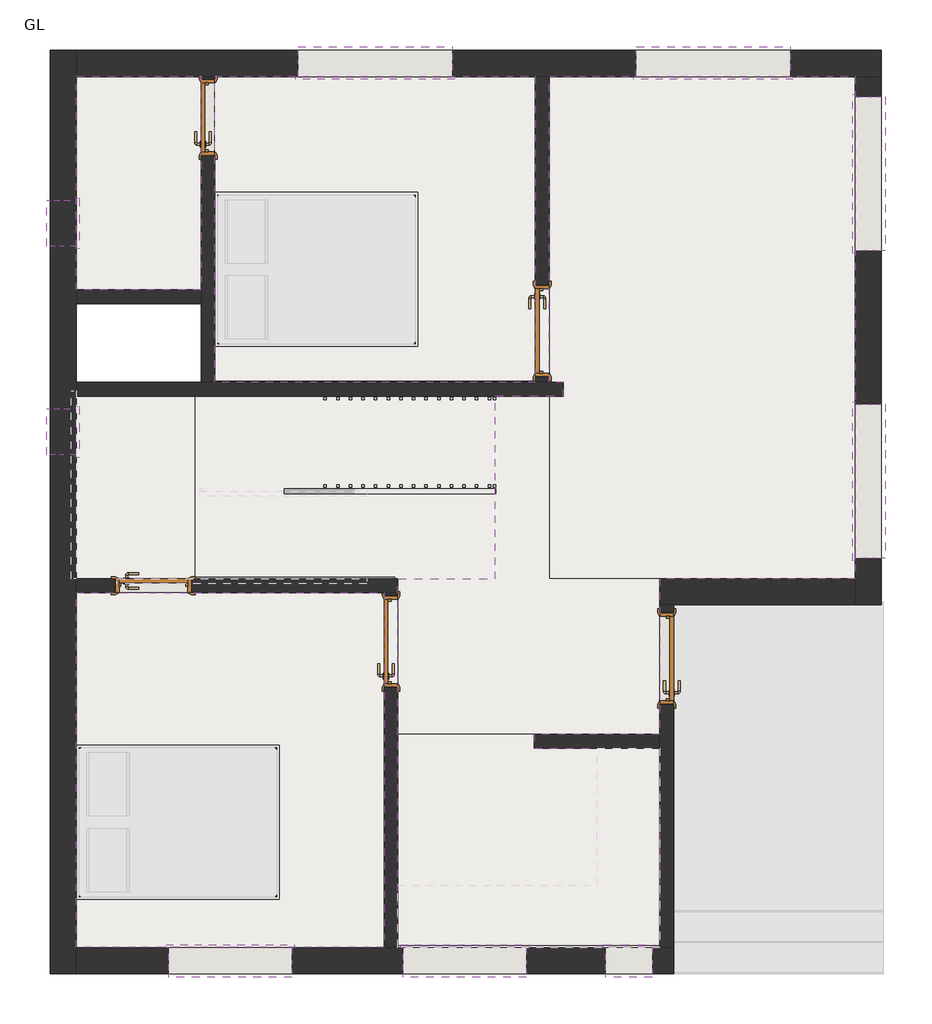
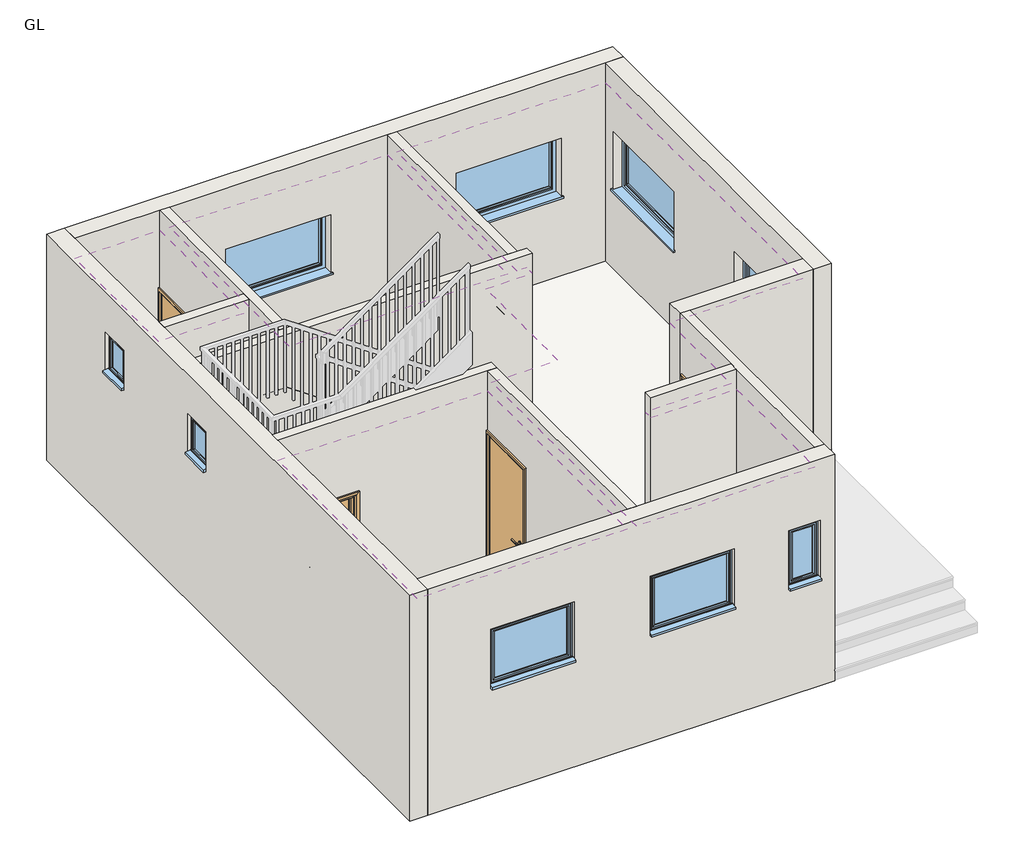
# One storey, part 1 of 2: 13 walls, 9 windows, 5 doors, 5 slabs, 4 coverings.
"""IFC4 building model written with IfcOpenShell, lengths in millimetres."""

from ifc_helpers import new_model, si_unit, frame, origin, origin_with_axes, place, context, project, spatial, polyline, outline, extrude, faceted_brep, transform, mapped, element, save
from components import doors_intsgl_d1_00c56c0f, doors_intsgl_d1_0ae72840, doors_intsgl_d2_4a296642, windows_sgl_plain_1219x910mm_2_5c67ae2b, windows_sgl_plain_w1_a675e60d, windows_sgl_plain_w3_7aa8ff83, windows_sgl_plain_w4_7e877f05

model = new_model("IFC4")

# Units and contexts
model_context = context("Model", 3, world=origin())
ifc_project = project(units=[si_unit("LENGTHUNIT", "METRE", prefix="MILLI")], contexts=[model_context])

# Site, building, storey
site = spatial("IfcSite", under=ifc_project)
building = spatial("IfcBuilding", under=site)
storey = spatial("IfcBuildingStorey", under=building, Name="GL", Elevation=0.0)

# Coverings
placement = place(None, origin())
element("IfcCovering", 1, ObjectType="Plain", at=placement, inside=storey, context=model_context, shape_type="SweptSolid", body=[
    extrude(outline(polyline([(-9804.9104231, 8478.0271174), (-11039.3504231, 8478.0271174), (-11039.3504231, 10590.7006314), (-9804.9104231, 10590.7006314), (-9804.9104231, 8478.0271174)])), frame((0.0, 0.0, 2743.2), z_axis=(0.0, 0.0, 1.0), x_axis=(1.0, 0.0, 0.0)), (0.0, 0.0, 1.0), 57.0),
])
element("IfcCovering", 2, ObjectType="Plain", at=placement, inside=storey, context=model_context, shape_type="SweptSolid", body=[
    extrude(outline(polyline([(-9667.7504231, 10590.7006314), (-6495.2904231, 10590.7006314), (-6495.2904231, 7563.6271174), (-9667.7504231, 7563.6271174), (-9667.7504231, 10590.7006314)])), frame((0.0, 0.0, 2743.2), z_axis=(0.0, 0.0, 1.0), x_axis=(1.0, 0.0, 0.0)), (0.0, 0.0, 1.0), 57.0),
])
element("IfcCovering", 3, ObjectType="Plain", at=placement, inside=storey, context=model_context, shape_type="SweptSolid", body=[
    extrude(outline(polyline([(-11039.3504231, 1964.8606314), (-11039.3504231, 5477.6191611), (-7992.723883, 5477.6191611), (-7992.723883, 1964.8606314), (-11039.3504231, 1964.8606314)])), frame((0.0, 0.0, 2743.2), z_axis=(0.0, 0.0, 1.0), x_axis=(1.0, 0.0, 0.0)), (0.0, 0.0, 1.0), 57.0),
])
element("IfcCovering", 4, ObjectType="Plain", at=placement, inside=storey, context=model_context, shape_type="SweptSolid", body=[
    extrude(outline(polyline([(-7855.563883, 1964.8606314), (-7855.563883, 5614.7791611), (-6892.1428068, 5614.7791611), (-6892.1428068, 7426.4671174), (-6216.8499038, 7426.4671174), (-6216.8499038, 7563.6271174), (-6358.1304231, 7563.6271174), (-6358.1304231, 10590.7006314), (-3327.9104231, 10590.7006314), (-3327.9104231, 5618.7656226), (-5262.223883, 5618.7656226), (-5262.223883, 4077.4180989), (-6506.823883, 4077.4180989), (-6506.823883, 3940.2580989), (-5262.223883, 3940.2580989), (-5262.223883, 1964.8606314), (-7855.563883, 1964.8606314)])), frame((0.0, 0.0, 2743.2), z_axis=(0.0, 0.0, 1.0), x_axis=(1.0, 0.0, 0.0)), (0.0, 0.0, 1.0), 57.0),
])

# Doors
doors_intsgl_d1_shape = doors_intsgl_d1_00c56c0f(model_context)
element("IfcDoor", 5, ObjectType="Doors_IntSgl : D1", at=placement, inside=storey, context=model_context, shape_type="MappedRepresentation", body=[
    mapped(doors_intsgl_d1_shape, transform((-6426.7104231, 8071.6271174, 0.0), x_axis=(0.0, -1.0, 0.0), y_axis=(1.0, 0.0, 0.0), z_axis=(0.0, 0.0, 1.0))),
])
element("IfcDoor", 6, ObjectType="Doors_IntSgl : D1", at=placement, inside=storey, context=model_context, shape_type="MappedRepresentation", body=[
    mapped(doors_intsgl_d1_shape, transform((-5193.643883, 4826.2856226, 0.0), x_axis=(0.0, 1.0, 0.0), y_axis=(-1.0, 0.0, 0.0), z_axis=(0.0, 0.0, 1.0))),
])
doors_intsgl_d1_2_shape = doors_intsgl_d1_0ae72840(model_context)
element("IfcDoor", 7, ObjectType="Doors_IntSgl : D1", at=placement, inside=storey, context=model_context, shape_type="MappedRepresentation", body=[
    mapped(doors_intsgl_d1_2_shape, transform((-7924.143883, 4995.0191611, 0.0), x_axis=(0.0, 1.0, 0.0), y_axis=(-1.0, 0.0, 0.0), z_axis=(0.0, 0.0, 1.0))),
])
doors_intsgl_d2_shape = doors_intsgl_d2_4a296642(model_context)
element("IfcDoor", 8, ObjectType="Doors_IntSgl : D2", at=placement, inside=storey, context=model_context, shape_type="MappedRepresentation", body=[
    mapped(doors_intsgl_d2_shape, transform((-10277.3504231, 5546.1991611, 0.0), x_axis=(1.0, 0.0, 0.0), y_axis=(0.0, 1.0, 0.0), z_axis=(0.0, 0.0, 1.0))),
])
element("IfcDoor", 9, ObjectType="Doors_IntSgl : D2", at=placement, inside=storey, context=model_context, shape_type="MappedRepresentation", body=[
    mapped(doors_intsgl_d2_shape, transform((-9736.3304231, 10185.6856226, 0.0), x_axis=(0.0, 1.0, 0.0), y_axis=(-1.0, 0.0, 0.0), z_axis=(0.0, 0.0, 1.0))),
])

# Slabs
element("IfcSlab", 10, ObjectType="BEDROOM FLOOR", at=placement, inside=storey, context=model_context, shape_type="SweptSolid", body=[
    extrude(outline(polyline([(-6358.1304231, 10590.7006314), (-6358.1304231, 7579.4271174), (-9667.7504231, 7579.4271174), (-9667.7504231, 10590.7006314), (-6358.1304231, 10590.7006314)])), origin_with_axes(), (0.0, 0.0, 1.0), 149.9616),
    extrude(outline(polyline([(-7855.563883, 5477.6191611), (-7855.563883, 1964.8606314), (-11039.3504231, 1964.8606314), (-11039.3504231, 5477.6191611), (-7855.563883, 5477.6191611)])), origin_with_axes(), (0.0, 0.0, 1.0), 149.9616),
])
element("IfcSlab", 11, ObjectType="FOYER", at=placement, inside=storey, context=model_context, shape_type="SweptSolid", body=[
    extrude(outline(polyline([(-5262.223883, 4077.4180989), (-7880.1504231, 4077.4180989), (-7880.1504231, 5634.7791611), (-9861.3504231, 5634.7791611), (-9861.3504231, 7426.4671174), (-6358.1304231, 7426.4671174), (-6358.1304231, 5618.7656226), (-5262.223883, 5618.7656226), (-5262.223883, 4077.4180989)])), frame((0.0, 0.0, -149.9616), z_axis=(0.0, 0.0, 1.0), x_axis=(1.0, 0.0, 0.0)), (0.0, 0.0, 1.0), 149.9616),
])
element("IfcSlab", 12, ObjectType="KITCHEN FLOOR", at=placement, inside=storey, context=model_context, shape_type="SweptSolid", body=[
    extrude(outline(polyline([(-7855.563883, 1989.8606314), (-7855.563883, 4077.4180989), (-5262.223883, 4077.4180989), (-5262.223883, 1989.8606314), (-7855.563883, 1989.8606314)])), frame((0.0, 0.0, -149.9616), z_axis=(0.0, 0.0, 1.0), x_axis=(1.0, 0.0, 0.0)), (0.0, 0.0, 1.0), 149.9616),
])
element("IfcSlab", 13, ObjectType="LIVING AND DINING AREA", at=placement, inside=storey, context=model_context, shape_type="SweptSolid", body=[
    extrude(outline(polyline([(-3327.9104231, 10590.7006314), (-3327.9104231, 5618.7656226), (-6358.1304231, 5618.7656226), (-6358.1304231, 10590.7006314), (-3327.9104231, 10590.7006314)])), frame((0.0, 0.0, -149.9616), z_axis=(0.0, 0.0, 1.0), x_axis=(1.0, 0.0, 0.0)), (0.0, 0.0, 1.0), 149.9616),
])
element("IfcSlab", 14, ObjectType="TOILET FLOOR", at=placement, inside=storey, context=model_context, shape_type="SweptSolid", body=[
    extrude(outline(polyline([(-9667.7504231, 10590.7006314), (-9667.7504231, 8478.0271174), (-11039.3504231, 8478.0271174), (-11039.3504231, 10590.7006314), (-9667.7504231, 10590.7006314)])), frame((0.0, 0.0, -149.9616), z_axis=(0.0, 0.0, 1.0), x_axis=(1.0, 0.0, 0.0)), (0.0, 0.0, 1.0), 149.9616),
    extrude(outline(polyline([(-9861.3504231, 7426.4671174), (-9861.3504231, 5477.6191611), (-11039.3504231, 5477.6191611), (-11039.3504231, 7426.4671174), (-9861.3504231, 7426.4671174)])), frame((0.0, 0.0, -149.9616), z_axis=(0.0, 0.0, 1.0), x_axis=(1.0, 0.0, 0.0)), (0.0, 0.0, 1.0), 149.9616),
])

# Walls
element("IfcWall", 15, ObjectType="EX WALL", at=placement, inside=storey, context=model_context, shape_type="Brep", body=[
    faceted_brep([(-11298.4304231, 10849.7806314, -426.72), (-11298.4304231, 1705.7806314, -426.72), (-11298.4304231, 1705.7806314, 3048.0), (-11298.4304231, 10849.7806314, 3048.0), (-11298.4304231, 6842.2671174, 2438.4), (-11298.4304231, 6842.2671174, 1828.8), (-11298.4304231, 7299.4671174, 1828.8), (-11298.4304231, 7299.4671174, 2438.4), (-11298.4304231, 8909.8271174, 2438.4), (-11298.4304231, 8909.8271174, 1828.8), (-11298.4304231, 9367.0271174, 1828.8), (-11298.4304231, 9367.0271174, 2438.4), (-11039.3504231, 10849.7806314, -426.72), (-11039.3504231, 10849.7806314, 3048.0), (-11039.3504231, 10590.7006314, 3048.0), (-11039.3504231, 8478.0271174, 3048.0), (-11039.3504231, 8340.8671174, 3048.0), (-11039.3504231, 7563.6271174, 3048.0), (-11039.3504231, 7426.4671174, 3048.0), (-11039.3504231, 5614.7791611, 3048.0), (-11039.3504231, 5477.6191611, 3048.0), (-11039.3504231, 1964.8606314, 3048.0), (-11039.3504231, 1705.7806314, 3048.0), (-11039.3504231, 1705.7806314, -426.72), (-11039.3504231, 1964.8606314, -426.72), (-11039.3504231, 5477.6191611, -426.72), (-11039.3504231, 5614.7791611, -426.72), (-11039.3504231, 7426.4671174, -426.72), (-11039.3504231, 7563.6271174, -426.72), (-11039.3504231, 8340.8671174, -426.72), (-11039.3504231, 8478.0271174, -426.72), (-11039.3504231, 10590.7006314, -426.72), (-11039.3504231, 6842.2671174, 2438.4), (-11039.3504231, 7299.4671174, 2438.4), (-11039.3504231, 7299.4671174, 1828.8), (-11039.3504231, 6842.2671174, 1828.8), (-11039.3504231, 8909.8271174, 2438.4), (-11039.3504231, 9367.0271174, 2438.4), (-11039.3504231, 9367.0271174, 1828.8), (-11039.3504231, 8909.8271174, 1828.8)], [[[0, 1, 2, 3], [4, 5, 6, 7], [8, 9, 10, 11]], [[12, 13, 14, 15, 16, 17, 18, 19, 20, 21, 22, 23, 24, 25, 26, 27, 28, 29, 30, 31], [32, 33, 34, 35], [36, 37, 38, 39]], [[1, 0, 12, 31, 30, 29, 28, 27, 26, 25, 24, 23]], [[3, 2, 22, 21, 20, 19, 18, 17, 16, 15, 14, 13]], [[2, 1, 23, 22]], [[0, 3, 13, 12]], [[5, 4, 32, 35]], [[6, 5, 35, 34]], [[7, 6, 34, 33]], [[4, 7, 33, 32]], [[9, 8, 36, 39]], [[10, 9, 39, 38]], [[11, 10, 38, 37]], [[8, 11, 37, 36]]]),
])
element("IfcWall", 16, ObjectType="EX WALL", at=placement, inside=storey, context=model_context, shape_type="Brep", body=[
    faceted_brep([(-5125.063883, 1964.8606314, -426.72), (-5262.223883, 1964.8606314, -426.72), (-7855.563883, 1964.8606314, -426.72), (-7992.723883, 1964.8606314, -426.72), (-11039.3504231, 1964.8606314, -426.72), (-11039.3504231, 1964.8606314, 3048.0), (-7992.723883, 1964.8606314, 3048.0), (-7855.563883, 1964.8606314, 3048.0), (-5262.223883, 1964.8606314, 3048.0), (-5125.063883, 1964.8606314, 3048.0), (-8906.4371531, 1964.8606314, 2110.0), (-10125.6371531, 1964.8606314, 2110.0), (-10125.6371531, 1964.8606314, 1200.0), (-8906.4371531, 1964.8606314, 1200.0), (-6585.563883, 1964.8606314, 2110.0), (-7804.763883, 1964.8606314, 2110.0), (-7804.763883, 1964.8606314, 1200.0), (-6585.563883, 1964.8606314, 1200.0), (-5338.423883, 1964.8606314, 2110.0), (-5795.623883, 1964.8606314, 2110.0), (-5795.623883, 1964.8606314, 1200.0), (-5338.423883, 1964.8606314, 1200.0), (-5125.063883, 1705.7806314, -426.72), (-5125.063883, 1705.7806314, 3048.0), (-11039.3504231, 1705.7806314, 3048.0), (-11039.3504231, 1705.7806314, -426.72), (-8906.4371531, 1705.7806314, 2110.0), (-8906.4371531, 1705.7806314, 1200.0), (-10125.6371531, 1705.7806314, 1200.0), (-10125.6371531, 1705.7806314, 2110.0), (-6585.563883, 1705.7806314, 2110.0), (-6585.563883, 1705.7806314, 1200.0), (-7804.763883, 1705.7806314, 1200.0), (-7804.763883, 1705.7806314, 2110.0), (-5338.423883, 1705.7806314, 2110.0), (-5338.423883, 1705.7806314, 1200.0), (-5795.623883, 1705.7806314, 1200.0), (-5795.623883, 1705.7806314, 2110.0)], [[[0, 1, 2, 3, 4, 5, 6, 7, 8, 9], [10, 11, 12, 13], [14, 15, 16, 17], [18, 19, 20, 21]], [[22, 23, 24, 25], [26, 27, 28, 29], [30, 31, 32, 33], [34, 35, 36, 37]], [[4, 3, 2, 1, 0, 22, 25]], [[9, 8, 7, 6, 5, 24, 23]], [[5, 4, 25, 24]], [[0, 9, 23, 22]], [[27, 26, 10, 13]], [[28, 27, 13, 12]], [[29, 28, 12, 11]], [[26, 29, 11, 10]], [[31, 30, 14, 17]], [[32, 31, 17, 16]], [[33, 32, 16, 15]], [[30, 33, 15, 14]], [[35, 34, 18, 21]], [[36, 35, 21, 20]], [[37, 36, 20, 19]], [[34, 37, 19, 18]]]),
])
element("IfcWall", 17, ObjectType="EX WALL", at=placement, inside=storey, context=model_context, shape_type="Brep", body=[
    faceted_brep([(-11039.3504231, 10590.7006314, -426.72), (-9804.9104231, 10590.7006314, -426.72), (-9667.7504231, 10590.7006314, -426.72), (-6495.2904231, 10590.7006314, -426.72), (-6358.1304231, 10590.7006314, -426.72), (-3327.9104231, 10590.7006314, -426.72), (-3068.8304231, 10590.7006314, -426.72), (-3068.8304231, 10590.7006314, 3048.0), (-3327.9104231, 10590.7006314, 3048.0), (-6358.1304231, 10590.7006314, 3048.0), (-6495.2904231, 10590.7006314, 3048.0), (-9667.7504231, 10590.7006314, 3048.0), (-9804.9104231, 10590.7006314, 3048.0), (-11039.3504231, 10590.7006314, 3048.0), (-8843.5204231, 10590.7006314, 2110.0), (-7319.5204231, 10590.7006314, 2110.0), (-7319.5204231, 10590.7006314, 1200.0), (-8843.5204231, 10590.7006314, 1200.0), (-5494.5304231, 10590.7006314, 2110.0), (-3970.5304231, 10590.7006314, 2110.0), (-3970.5304231, 10590.7006314, 1200.0), (-5494.5304231, 10590.7006314, 1200.0), (-11039.3504231, 10849.7806314, -426.72), (-11039.3504231, 10849.7806314, 3048.0), (-3068.8304231, 10849.7806314, 3048.0), (-3068.8304231, 10849.7806314, -426.72), (-8843.5204231, 10849.7806314, 2110.0), (-8843.5204231, 10849.7806314, 1200.0), (-7319.5204231, 10849.7806314, 1200.0), (-7319.5204231, 10849.7806314, 2110.0), (-5494.5304231, 10849.7806314, 2110.0), (-5494.5304231, 10849.7806314, 1200.0), (-3970.5304231, 10849.7806314, 1200.0), (-3970.5304231, 10849.7806314, 2110.0)], [[[0, 1, 2, 3, 4, 5, 6, 7, 8, 9, 10, 11, 12, 13], [14, 15, 16, 17], [18, 19, 20, 21]], [[22, 23, 24, 25], [26, 27, 28, 29], [30, 31, 32, 33]], [[6, 5, 4, 3, 2, 1, 0, 22, 25]], [[13, 12, 11, 10, 9, 8, 7, 24, 23]], [[0, 13, 23, 22]], [[7, 6, 25, 24]], [[27, 26, 14, 17]], [[28, 27, 17, 16]], [[29, 28, 16, 15]], [[26, 29, 15, 14]], [[31, 30, 18, 21]], [[32, 31, 21, 20]], [[33, 32, 20, 19]], [[30, 33, 19, 18]]]),
])
element("IfcWall", 18, ObjectType="EX WALL", at=placement, inside=storey, context=model_context, shape_type="Brep", body=[
    faceted_brep([(-3327.9104231, 10590.7006314, -426.72), (-3327.9104231, 5618.7656226, -426.72), (-3327.9104231, 5359.6856226, -426.72), (-3327.9104231, 5359.6856226, 3048.0), (-3327.9104231, 5618.7656226, 3048.0), (-3327.9104231, 10590.7006314, 3048.0), (-3327.9104231, 10388.8856226, 2110.0), (-3327.9104231, 8864.8856226, 2110.0), (-3327.9104231, 8864.8856226, 1200.0), (-3327.9104231, 10388.8856226, 1200.0), (-3327.9104231, 7345.9656226, 2110.0), (-3327.9104231, 5821.9656226, 2110.0), (-3327.9104231, 5821.9656226, 1200.0), (-3327.9104231, 7345.9656226, 1200.0), (-3068.8304231, 10590.7006314, -426.72), (-3068.8304231, 10590.7006314, 3048.0), (-3068.8304231, 5359.6856226, 3048.0), (-3068.8304231, 5359.6856226, -426.72), (-3068.8304231, 10388.8856226, 2110.0), (-3068.8304231, 10388.8856226, 1200.0), (-3068.8304231, 8864.8856226, 1200.0), (-3068.8304231, 8864.8856226, 2110.0), (-3068.8304231, 7345.9656226, 2110.0), (-3068.8304231, 7345.9656226, 1200.0), (-3068.8304231, 5821.9656226, 1200.0), (-3068.8304231, 5821.9656226, 2110.0)], [[[0, 1, 2, 3, 4, 5], [6, 7, 8, 9], [10, 11, 12, 13]], [[14, 15, 16, 17], [18, 19, 20, 21], [22, 23, 24, 25]], [[2, 1, 0, 14, 17]], [[5, 4, 3, 16, 15]], [[0, 5, 15, 14]], [[3, 2, 17, 16]], [[19, 18, 6, 9]], [[20, 19, 9, 8]], [[21, 20, 8, 7]], [[18, 21, 7, 6]], [[23, 22, 10, 13]], [[24, 23, 13, 12]], [[25, 24, 12, 11]], [[22, 25, 11, 10]]]),
])
element("IfcWall", 19, ObjectType="EX WALL", at=placement, inside=storey, context=model_context, shape_type="Brep", body=[
    faceted_brep([(-3327.9104231, 5618.7656226, -426.72), (-5262.223883, 5618.7656226, -426.72), (-5262.223883, 5618.7656226, 3048.0), (-3327.9104231, 5618.7656226, 3048.0), (-3327.9104231, 5359.6856226, -426.72), (-3327.9104231, 5359.6856226, 3048.0), (-5125.063883, 5359.6856226, 3048.0), (-5262.223883, 5359.6856226, 3048.0), (-5262.223883, 5359.6856226, -426.72), (-5125.063883, 5359.6856226, -426.72)], [[[0, 1, 2, 3]], [[4, 5, 6, 7, 8, 9]], [[1, 0, 4, 9, 8]], [[3, 2, 7, 6, 5]], [[0, 3, 5, 4]], [[2, 1, 8, 7]]]),
])
element("IfcWall", 20, ObjectType="IN WALL", at=placement, inside=storey, context=model_context, shape_type="SweptSolid", body=[
    extrude(outline(polyline([(10590.7006314, -426.72), (7563.6271174, -426.72), (7563.6271174, 3048.0), (10590.7006314, 3048.0), (10590.7006314, -426.72)]), holes=[polyline([(7614.4271174, 2110.0), (7614.4271174, 0.0), (8528.8271174, 0.0), (8528.8271174, 2110.0), (7614.4271174, 2110.0)])]), frame((-6495.2904231, 0.0, 0.0), z_axis=(1.0, 0.0, 0.0), x_axis=(0.0, 1.0, 0.0)), (0.0, 0.0, 1.0), 137.16),
])
element("IfcWall", 21, ObjectType="IN WALL", at=placement, inside=storey, context=model_context, shape_type="Brep", body=[
    faceted_brep([(-6216.8499038, 7563.6271174, -426.72), (-6358.1304231, 7563.6271174, -426.72), (-6495.2904231, 7563.6271174, -426.72), (-9667.7504231, 7563.6271174, -426.72), (-9804.9104231, 7563.6271174, -426.72), (-11039.3504231, 7563.6271174, -426.72), (-11039.3504231, 7563.6271174, 3048.0), (-9804.9104231, 7563.6271174, 3048.0), (-9667.7504231, 7563.6271174, 3048.0), (-6495.2904231, 7563.6271174, 3048.0), (-6358.1304231, 7563.6271174, 3048.0), (-6216.8499038, 7563.6271174, 3048.0), (-6216.8499038, 7426.4671174, -426.72), (-6216.8499038, 7426.4671174, 3048.0), (-11039.3504231, 7426.4671174, 3048.0), (-11039.3504231, 7426.4671174, -426.72)], [[[0, 1, 2, 3, 4, 5, 6, 7, 8, 9, 10, 11]], [[12, 13, 14, 15]], [[5, 4, 3, 2, 1, 0, 12, 15]], [[11, 10, 9, 8, 7, 6, 14, 13]], [[0, 11, 13, 12]], [[6, 5, 15, 14]]]),
])
element("IfcWall", 22, ObjectType="IN WALL", at=placement, inside=storey, context=model_context, shape_type="Brep", body=[
    faceted_brep([(-9667.7504231, 7563.6271174, -426.72), (-9667.7504231, 10590.7006314, -426.72), (-9667.7504231, 10590.7006314, 3048.0), (-9667.7504231, 7563.6271174, 3048.0), (-9667.7504231, 10566.6856226, 1828.8), (-9667.7504231, 10566.6856226, 0.0), (-9667.7504231, 9804.6856226, 0.0), (-9667.7504231, 9804.6856226, 1828.8), (-9804.9104231, 10590.7006314, -426.72), (-9804.9104231, 8478.0271174, -426.72), (-9804.9104231, 8340.8671174, -426.72), (-9804.9104231, 7563.6271174, -426.72), (-9804.9104231, 7563.6271174, 3048.0), (-9804.9104231, 8340.8671174, 3048.0), (-9804.9104231, 8478.0271174, 3048.0), (-9804.9104231, 10590.7006314, 3048.0), (-9804.9104231, 10566.6856226, 0.0), (-9804.9104231, 10566.6856226, 1828.8), (-9804.9104231, 9804.6856226, 1828.8), (-9804.9104231, 9804.6856226, 0.0)], [[[0, 1, 2, 3], [4, 5, 6, 7]], [[8, 9, 10, 11, 12, 13, 14, 15], [16, 17, 18, 19]], [[1, 0, 11, 10, 9, 8]], [[3, 2, 15, 14, 13, 12]], [[2, 1, 8, 15]], [[0, 3, 12, 11]], [[16, 5, 4, 17]], [[17, 4, 7, 18]], [[18, 7, 6, 19]], [[5, 16, 19, 6]]]),
])
element("IfcWall", 23, ObjectType="IN WALL", at=placement, inside=storey, context=model_context, shape_type="SweptSolid", body=[
    extrude(outline(polyline([(-9804.9104231, 8340.8671174), (-11039.3504231, 8340.8671174), (-11039.3504231, 8478.0271174), (-9804.9104231, 8478.0271174), (-9804.9104231, 8340.8671174)])), frame((0.0, 0.0, -426.72), z_axis=(0.0, 0.0, 1.0), x_axis=(1.0, 0.0, 0.0)), (0.0, 0.0, 1.0), 3474.72),
])
element("IfcWall", 24, ObjectType="IN WALL", at=placement, inside=storey, context=model_context, shape_type="Brep", body=[
    faceted_brep([(-11039.3504231, 5477.6191611, -426.72), (-7992.723883, 5477.6191611, -426.72), (-7855.563883, 5477.6191611, -426.72), (-7855.563883, 5477.6191611, 3048.0), (-7992.723883, 5477.6191611, 3048.0), (-11039.3504231, 5477.6191611, 3048.0), (-9896.3504231, 5477.6191611, 1828.8), (-9896.3504231, 5477.6191611, 0.0), (-10658.3504231, 5477.6191611, 0.0), (-10658.3504231, 5477.6191611, 1828.8), (-7855.563883, 5614.7791611, -426.72), (-11039.3504231, 5614.7791611, -426.72), (-11039.3504231, 5614.7791611, 3048.0), (-7855.563883, 5614.7791611, 3048.0), (-9896.3504231, 5614.7791611, 0.0), (-9896.3504231, 5614.7791611, 1828.8), (-10658.3504231, 5614.7791611, 1828.8), (-10658.3504231, 5614.7791611, 0.0)], [[[0, 1, 2, 3, 4, 5], [6, 7, 8, 9]], [[10, 11, 12, 13], [14, 15, 16, 17]], [[2, 1, 0, 11, 10]], [[5, 4, 3, 13, 12]], [[0, 5, 12, 11]], [[3, 2, 10, 13]], [[14, 7, 6, 15]], [[15, 6, 9, 16]], [[16, 9, 8, 17]], [[7, 14, 17, 8]]]),
])
element("IfcWall", 25, ObjectType="IN WALL", at=placement, inside=storey, context=model_context, shape_type="SweptSolid", body=[
    extrude(outline(polyline([(5477.6191611, -426.72), (1964.8606314, -426.72), (1964.8606314, 3048.0), (5477.6191611, 3048.0), (5477.6191611, -426.72)]), holes=[polyline([(5452.2191611, 0.0), (5452.2191611, 2110.0), (4537.8191611, 2110.0), (4537.8191611, 0.0), (5452.2191611, 0.0)])]), frame((-7992.723883, 0.0, 0.0), z_axis=(1.0, 0.0, 0.0), x_axis=(0.0, 1.0, 0.0)), (0.0, 0.0, 1.0), 137.16),
])
element("IfcWall", 26, ObjectType="IN WALL", at=placement, inside=storey, context=model_context, shape_type="Brep", body=[
    faceted_brep([(-5125.063883, 1964.8606314, -426.72), (-5125.063883, 5359.6856226, -426.72), (-5125.063883, 5359.6856226, 3048.0), (-5125.063883, 1964.8606314, 3048.0), (-5125.063883, 5283.4856226, 2110.0), (-5125.063883, 5283.4856226, 0.0), (-5125.063883, 4369.0856226, 0.0), (-5125.063883, 4369.0856226, 2110.0), (-5262.223883, 5359.6856226, -426.72), (-5262.223883, 4077.4180989, -426.72), (-5262.223883, 3940.2580989, -426.72), (-5262.223883, 1964.8606314, -426.72), (-5262.223883, 1964.8606314, 3048.0), (-5262.223883, 3940.2580989, 3048.0), (-5262.223883, 4077.4180989, 3048.0), (-5262.223883, 5359.6856226, 3048.0), (-5262.223883, 5283.4856226, 0.0), (-5262.223883, 5283.4856226, 2110.0), (-5262.223883, 4369.0856226, 2110.0), (-5262.223883, 4369.0856226, 0.0)], [[[0, 1, 2, 3], [4, 5, 6, 7]], [[8, 9, 10, 11, 12, 13, 14, 15], [16, 17, 18, 19]], [[1, 0, 11, 10, 9, 8]], [[3, 2, 15, 14, 13, 12]], [[0, 3, 12, 11]], [[2, 1, 8, 15]], [[16, 5, 4, 17]], [[17, 4, 7, 18]], [[18, 7, 6, 19]], [[5, 16, 19, 6]]]),
])
element("IfcWall", 27, ObjectType="IN WALL", at=placement, inside=storey, context=model_context, shape_type="SweptSolid", body=[
    extrude(outline(polyline([(-6506.823883, 4077.4180989), (-5262.223883, 4077.4180989), (-5262.223883, 3940.2580989), (-6506.823883, 3940.2580989), (-6506.823883, 4077.4180989)])), frame((0.0, 0.0, -426.72), z_axis=(0.0, 0.0, 1.0), x_axis=(1.0, 0.0, 0.0)), (0.0, 0.0, 1.0), 3474.72),
])

# Windows
windows_sgl_plain_1219x910mm_2_shape = windows_sgl_plain_1219x910mm_2_5c67ae2b(model_context)
element("IfcWindow", 28, ObjectType="Windows_Sgl_Plain : 1219x910mm 2", at=placement, inside=storey, context=model_context, shape_type="MappedRepresentation", body=[
    mapped(windows_sgl_plain_1219x910mm_2_shape, transform((-9516.0371531, 1843.7771992, 0.0), x_axis=(-1.0, 0.0, 0.0), y_axis=(0.0, -1.0, 0.0), z_axis=(0.0, 0.0, 1.0))),
])
element("IfcWindow", 29, ObjectType="Windows_Sgl_Plain : 1219x910mm 2", at=placement, inside=storey, context=model_context, shape_type="MappedRepresentation", body=[
    mapped(windows_sgl_plain_1219x910mm_2_shape, transform((-7195.163883, 1843.7771992, 0.0), x_axis=(-1.0, 0.0, 0.0), y_axis=(0.0, -1.0, 0.0), z_axis=(0.0, 0.0, 1.0))),
])
windows_sgl_plain_w1_shape = windows_sgl_plain_w1_a675e60d(model_context)
element("IfcWindow", 30, ObjectType="Windows_Sgl_Plain : W1", at=placement, inside=storey, context=model_context, shape_type="MappedRepresentation", body=[
    mapped(windows_sgl_plain_w1_shape, transform((-8081.5204231, 10711.7840636, 0.0), x_axis=(1.0, 0.0, 0.0), y_axis=(0.0, 1.0, 0.0), z_axis=(0.0, 0.0, 1.0))),
])
element("IfcWindow", 31, ObjectType="Windows_Sgl_Plain : W1", at=placement, inside=storey, context=model_context, shape_type="MappedRepresentation", body=[
    mapped(windows_sgl_plain_w1_shape, transform((-4732.5304231, 10711.7840636, 0.0), x_axis=(1.0, 0.0, 0.0), y_axis=(0.0, 1.0, 0.0), z_axis=(0.0, 0.0, 1.0))),
])
element("IfcWindow", 32, ObjectType="Windows_Sgl_Plain : W1", at=placement, inside=storey, context=model_context, shape_type="MappedRepresentation", body=[
    mapped(windows_sgl_plain_w1_shape, transform((-3206.826991, 9626.8856226, 0.0), x_axis=(0.0, -1.0, 0.0), y_axis=(1.0, 0.0, 0.0), z_axis=(0.0, 0.0, 1.0))),
])
element("IfcWindow", 33, ObjectType="Windows_Sgl_Plain : W1", at=placement, inside=storey, context=model_context, shape_type="MappedRepresentation", body=[
    mapped(windows_sgl_plain_w1_shape, transform((-3206.826991, 6583.9656226, 0.0), x_axis=(0.0, -1.0, 0.0), y_axis=(1.0, 0.0, 0.0), z_axis=(0.0, 0.0, 1.0))),
])
windows_sgl_plain_w3_shape = windows_sgl_plain_w3_7aa8ff83(model_context)
element("IfcWindow", 34, ObjectType="Windows_Sgl_Plain : W3", at=placement, inside=storey, context=model_context, shape_type="MappedRepresentation", body=[
    mapped(windows_sgl_plain_w3_shape, transform((-5567.023883, 1843.7771992, 0.0), x_axis=(-1.0, 0.0, 0.0), y_axis=(0.0, -1.0, 0.0), z_axis=(0.0, 0.0, 1.0))),
])
windows_sgl_plain_w4_shape = windows_sgl_plain_w4_7e877f05(model_context)
element("IfcWindow", 35, ObjectType="Windows_Sgl_Plain : W4", at=placement, inside=storey, context=model_context, shape_type="MappedRepresentation", body=[
    mapped(windows_sgl_plain_w4_shape, transform((-11160.4338553, 7070.8671174, 328.4), x_axis=(0.0, 1.0, 0.0), y_axis=(-1.0, 0.0, 0.0), z_axis=(0.0, 0.0, 1.0))),
])
element("IfcWindow", 36, ObjectType="Windows_Sgl_Plain : W4", at=placement, inside=storey, context=model_context, shape_type="MappedRepresentation", body=[
    mapped(windows_sgl_plain_w4_shape, transform((-11160.4338553, 9138.4271174, 328.4), x_axis=(0.0, 1.0, 0.0), y_axis=(-1.0, 0.0, 0.0), z_axis=(0.0, 0.0, 1.0))),
])

save(model, "model.ifc")

# Revit data of these elements
# Type "Plain"
#   Keynote = "K40"
#   built-in parameter 1002203 = 1 (stored number, unit not read)
#   built-in parameter 1002202 = 1 (stored number, unit not read)
#   Layers, outside or top first: 0.147638 ft "Metal Stud Layer" (function 1); 0.03937 ft "Gypsum Wall Board" (function 1)
# Type "Doors_IntSgl : D1"
#   Type Mark = "46"
#   Type Comments = "Internal Single"
#   Operation = "SingleSwingRight"
#   Manufacturer = "Revit"
#   Keynote = "L20"
#   Description = "Internal Single Door"
#   Analytic Construction = "Metal"
#   UnderCut = 0.026247 ft
#   Tolerance = 0.006562 ft
#   Thickness = 0.124672 ft
#   Thermal Resistance (R) = 0.270117 (m²·K)/W
#   Structural Tolerance = 0.026247 ft
#   StopDepth = 0.104987 ft
#   Stop Thickness = 0.062336 ft
#   Rough Width = 3.0 ft
#   Rough Height = 6.922572 ft
#   Height to Top Lock Rail = 3.28084 ft
#   Heat Transfer Coefficient (U) = 3.7021 W/(m²·K)
#   Handle Z Distance = 2.952756 ft
#   Handle X Distance = 0.246063 ft
#   Frame Thickness = 0.104987 ft
#   Door Panel Width = 2.724409 ft
#   Door Panel Thickness = 0.124672 ft
#   Door Panel Offset = 0.0 ft
#   Height = 6.922572 ft
#   Width = 3.0 ft
#   Door Panel Height = 6.75853 ft
#   Architrave Setback = 0.016404 ft
#   Vis - Ironmongery = yes
#   Material Ironmongery = Door - Handle
#   Material Frame = Door - Frame/Mullion (1)
#   Material Door = Door - Panel
#   Material Architrave = Door - Architrave
#   Visual Light Transmittance = 0
#   Solar Heat Gain Coefficient = 0
#   Function = (empty or 0)
#   Wall Closure = (empty or 0)
# Type "Doors_IntSgl : D2"
#   Type Mark = "47"
#   Type Comments = "Internal Single"
#   Operation = "SingleSwingRight"
#   Manufacturer = "Revit"
#   Keynote = "L20"
#   Description = "Internal Single Door"
#   Analytic Construction = "Metal"
#   UnderCut = 0.026247 ft
#   Tolerance = 0.006562 ft
#   Thickness = 0.124672 ft
#   Thermal Resistance (R) = 0.270117 (m²·K)/W
#   Structural Tolerance = 0.026247 ft
#   StopDepth = 0.104987 ft
#   Stop Thickness = 0.062336 ft
#   Rough Width = 2.5 ft
#   Rough Height = 6.0 ft
#   Height to Top Lock Rail = 3.28084 ft
#   Heat Transfer Coefficient (U) = 3.7021 W/(m²·K)
#   Handle Z Distance = 2.952756 ft
#   Handle X Distance = 0.246063 ft
#   Frame Thickness = 0.104987 ft
#   Door Panel Width = 2.224409 ft
#   Door Panel Thickness = 0.124672 ft
#   Door Panel Offset = 0.0 ft
#   Height = 6.0 ft
#   Width = 2.5 ft
#   Door Panel Height = 5.835958 ft
#   Architrave Setback = 0.016404 ft
#   Vis - Ironmongery = yes
#   Material Ironmongery = Door - Handle
#   Material Frame = Door - Frame/Mullion (1)
#   Material Door = Door - Panel
#   Material Architrave = Door - Architrave
#   Visual Light Transmittance = 0
#   Solar Heat Gain Coefficient = 0
#   Function = (empty or 0)
#   Wall Closure = (empty or 0)
# Type "BEDROOM FLOOR"
#   Function = 0
#   Layers, outside or top first: 0.072 ft "Wood Sheathing, Chipboard" (function 5); 0.42 ft "Structure, Timber Joist/Rafter Layer" (function 1)
# Type "FOYER"
#   Function = 0
#   Layers, outside or top first: 0.072 ft "Wood Sheathing, Chipboard" (function 5); 0.42 ft "Structure, Timber Joist/Rafter Layer" (function 1)
# Type "KITCHEN FLOOR"
#   Function = 0
#   Layers, outside or top first: 0.072 ft "Wood Sheathing, Chipboard" (function 5); 0.42 ft "Structure, Timber Joist/Rafter Layer" (function 1)
# Type "LIVING AND DINING AREA"
#   Function = 0
#   Layers, outside or top first: 0.072 ft "Wood Sheathing, Chipboard" (function 5); 0.42 ft "Structure, Timber Joist/Rafter Layer" (function 1)
# Type "TOILET FLOOR"
#   Function = 0
#   Layers, outside or top first: 0.072 ft "Wood Sheathing, Chipboard" (function 5); 0.42 ft "Structure, Timber Joist/Rafter Layer" (function 1)
# Type "EX WALL"
#   Keynote = "F10"
#   Layers, outside or top first: 0.85 ft "Brick, Common" (function 1)
# Type "IN WALL"
#   Keynote = "F10"
#   Layers, outside or top first: 0.45 ft "Brick, Common" (function 1)
# Type "Windows_Sgl_Plain : 1219x910mm 2"
#   Type Mark = "61"
#   Operation = "SinglePanel"
#   Construction Type Id = "SGL"
#   Manufacturer = "Revit"
#   Keynote = "L10"
#   Analytic Construction = "Large single-glazed windows"
#   Wrap Layers (Ext) from Ext = 0.336286 ft
#   Wrap Layers (Int) from Ext = 0.582349 ft
#   Window Board Projection = 0.082021 ft
#   Window Board Extension = 0.082021 ft
#   Visual Light Transmittance = 0.9
#   Solar Heat Gain Coefficient = 0.86
#   Rough Width = 4.0 ft
#   Rough Height = 2.985564 ft
#   Height = 2.985564 ft
#   Width = 4.0 ft
#   Heat Transfer Coefficient (U) = 5.5617 W/(m²·K)
#   Glazing Thickness = 0.07874 ft
#   FrameOffset - External = 0.164042 ft
#   Frame Depth = 0.213255 ft
#   Default Head Height = 6.922572 ft
#   Cill Depth = 0.287073 ft
#   Cavity Closer Width = 0.164042 ft
#   Cavity Closer Offset from Ext = 0.336286 ft
#   Cavity Closer Depth = 0.278871 ft
#   Vis - Cavity Closers = yes
#   Define Thermal Properties by = 1
#   Material Trim = Window Frame
#   Material Glass = Glass
#   Material Frame = Window Frame
#   Wall Closure = (empty or 0)
# Type "Windows_Sgl_Plain : W1"
#   Type Mark = "60"
#   Operation = "SinglePanel"
#   Construction Type Id = "SGL"
#   Manufacturer = "Revit"
#   Keynote = "L10"
#   Analytic Construction = "Large single-glazed windows"
#   Wrap Layers (Ext) from Ext = 0.336286 ft
#   Wrap Layers (Int) from Ext = 0.582349 ft
#   Window Board Projection = 0.082021 ft
#   Window Board Extension = 0.082021 ft
#   Visual Light Transmittance = 0.9
#   Solar Heat Gain Coefficient = 0.86
#   Rough Width = 5.0 ft
#   Rough Height = 2.985564 ft
#   Height = 2.985564 ft
#   Width = 5.0 ft
#   Heat Transfer Coefficient (U) = 5.5617 W/(m²·K)
#   Glazing Thickness = 0.07874 ft
#   FrameOffset - External = 0.164042 ft
#   Frame Depth = 0.213255 ft
#   Default Head Height = 6.922572 ft
#   Cill Depth = 0.287073 ft
#   Cavity Closer Width = 0.164042 ft
#   Cavity Closer Offset from Ext = 0.336286 ft
#   Cavity Closer Depth = 0.278871 ft
#   Vis - Cavity Closers = yes
#   Define Thermal Properties by = 1
#   Material Trim = Window Frame
#   Material Glass = Glass
#   Material Frame = Window Frame
#   Wall Closure = (empty or 0)
# Type "Windows_Sgl_Plain : W3"
#   Type Mark = "58"
#   Operation = "SinglePanel"
#   Construction Type Id = "SGL"
#   Manufacturer = "Revit"
#   Keynote = "L10"
#   Analytic Construction = "Large single-glazed windows"
#   Wrap Layers (Ext) from Ext = 0.336286 ft
#   Wrap Layers (Int) from Ext = 0.582349 ft
#   Window Board Projection = 0.082021 ft
#   Window Board Extension = 0.082021 ft
#   Visual Light Transmittance = 0.9
#   Solar Heat Gain Coefficient = 0.86
#   Rough Width = 1.5 ft
#   Rough Height = 2.985564 ft
#   Height = 2.985564 ft
#   Width = 1.5 ft
#   Heat Transfer Coefficient (U) = 5.5617 W/(m²·K)
#   Glazing Thickness = 0.07874 ft
#   FrameOffset - External = 0.164042 ft
#   Frame Depth = 0.213255 ft
#   Default Head Height = 6.922572 ft
#   Cill Depth = 0.287073 ft
#   Cavity Closer Width = 0.164042 ft
#   Cavity Closer Offset from Ext = 0.336286 ft
#   Cavity Closer Depth = 0.278871 ft
#   Vis - Cavity Closers = yes
#   Define Thermal Properties by = 1
#   Material Trim = Window Frame
#   Material Glass = Glass
#   Material Frame = Window Frame
#   Wall Closure = (empty or 0)
# Type "Windows_Sgl_Plain : W4"
#   Type Mark = "59"
#   Operation = "SinglePanel"
#   Construction Type Id = "SGL"
#   Manufacturer = "Revit"
#   Keynote = "L10"
#   Analytic Construction = "Large single-glazed windows"
#   Wrap Layers (Ext) from Ext = 0.336286 ft
#   Wrap Layers (Int) from Ext = 0.582349 ft
#   Window Board Projection = 0.082021 ft
#   Window Board Extension = 0.082021 ft
#   Visual Light Transmittance = 0.9
#   Solar Heat Gain Coefficient = 0.86
#   Rough Width = 1.5 ft
#   Rough Height = 2.0 ft
#   Height = 2.0 ft
#   Width = 1.5 ft
#   Heat Transfer Coefficient (U) = 5.5617 W/(m²·K)
#   Glazing Thickness = 0.07874 ft
#   FrameOffset - External = 0.164042 ft
#   Frame Depth = 0.213255 ft
#   Default Head Height = 6.922572 ft
#   Cill Depth = 0.287073 ft
#   Cavity Closer Width = 0.164042 ft
#   Cavity Closer Offset from Ext = 0.336286 ft
#   Cavity Closer Depth = 0.278871 ft
#   Vis - Cavity Closers = yes
#   Define Thermal Properties by = 1
#   Material Trim = Window Frame
#   Material Glass = Glass
#   Material Frame = Window Frame
#   Wall Closure = (empty or 0)
# Elements 1, 2, 3, 4 (IfcCovering, "Plain")
#   Height Offset From Level = 9.0 ft
#   Phase Created = New Construction
#   Materials on its faces: "Gypsum Wall Board", "Metal Stud Layer"
# Elements 5, 6, 7 (IfcDoor, "Doors_IntSgl : D1")
#   Phase Created = New Construction
#   Materials on its faces: "Door - Architrave", "Door - Handle", "Door - Frame/Mullion (1)", "Door - Panel"
# Elements 8, 9 (IfcDoor, "Doors_IntSgl : D2")
#   Phase Created = New Construction
#   Materials on its faces: "Door - Architrave", "Door - Handle", "Door - Frame/Mullion (1)", "Door - Panel"
# Element 10 (IfcSlab, "BEDROOM FLOOR")
#   Height Offset From Level = 0.492 ft
#   Phase Created = New Construction
#   Materials on its faces: "Structure, Timber Joist/Rafter Layer", "Wood Sheathing, Chipboard"
# Element 11 (IfcSlab, "FOYER")
#   Height Offset From Level = 0.0 ft
#   Phase Created = New Construction
#   Materials on its faces: "Structure, Timber Joist/Rafter Layer", "Wood Sheathing, Chipboard"
# Element 12 (IfcSlab, "KITCHEN FLOOR")
#   built-in parameter 1001955 = 3.14159 (stored number, unit not read)
#   Height Offset From Level = 0.0 ft
#   Phase Created = New Construction
#   Materials on its faces: "Structure, Timber Joist/Rafter Layer", "Wood Sheathing, Chipboard"
# Element 13 (IfcSlab, "LIVING AND DINING AREA")
#   Height Offset From Level = 0.0 ft
#   Phase Created = New Construction
#   Materials on its faces: "Structure, Timber Joist/Rafter Layer", "Wood Sheathing, Chipboard"
# Element 14 (IfcSlab, "TOILET FLOOR")
#   Height Offset From Level = 0.0 ft
#   Phase Created = New Construction
#   Materials on its faces: "Structure, Timber Joist/Rafter Layer", "Wood Sheathing, Chipboard"
# Elements 15, 16, 17, 18, 19 (IfcWall, "EX WALL")
#   built-in parameter 1001111 = -1.4 ft
#   Top Offset = 0.0 ft
#   Base Offset = -1.4 ft
#   wall height = 11.4 ft
#   Phase Created = New Construction
#   Base Constraint = GL
#   Top Constraint = FFL
#   Materials on its faces: "Brick, Common"
# Elements 20, 21, 22, 23, 24, 25, 26, 27 (IfcWall, "IN WALL")
#   built-in parameter 1001111 = -1.4 ft
#   Top Offset = 0.0 ft
#   Base Offset = -1.4 ft
#   wall height = 11.4 ft
#   Phase Created = New Construction
#   Base Constraint = GL
#   Top Constraint = FFL
#   Materials on its faces: "Brick, Common"
# Element 28 (IfcWindow, "Windows_Sgl_Plain : 1219x910mm 2")
#   Mark = "5"
#   Phase Created = New Construction
#   Materials on its faces: "Window Frame", "Glass"
# Element 29 (IfcWindow, "Windows_Sgl_Plain : 1219x910mm 2")
#   Mark = "6"
#   Phase Created = New Construction
#   Materials on its faces: "Window Frame", "Glass"
# Element 30 (IfcWindow, "Windows_Sgl_Plain : W1")
#   Mark = "1"
#   Phase Created = New Construction
#   Materials on its faces: "Window Frame", "Glass"
# Element 31 (IfcWindow, "Windows_Sgl_Plain : W1")
#   Mark = "2"
#   Phase Created = New Construction
#   Materials on its faces: "Window Frame", "Glass"
# Element 32 (IfcWindow, "Windows_Sgl_Plain : W1")
#   Mark = "3"
#   Phase Created = New Construction
#   Materials on its faces: "Window Frame", "Glass"
# Element 33 (IfcWindow, "Windows_Sgl_Plain : W1")
#   Mark = "4"
#   Phase Created = New Construction
#   Materials on its faces: "Window Frame", "Glass"
# Element 34 (IfcWindow, "Windows_Sgl_Plain : W3")
#   Mark = "7"
#   Phase Created = New Construction
#   Materials on its faces: "Window Frame", "Glass"
# Element 35 (IfcWindow, "Windows_Sgl_Plain : W4")
#   Mark = "8"
#   Phase Created = New Construction
#   Materials on its faces: "Window Frame", "Glass"
# Element 36 (IfcWindow, "Windows_Sgl_Plain : W4")
#   Mark = "9"
#   Phase Created = New Construction
#   Materials on its faces: "Window Frame", "Glass"
# Materials
#   "Metal Stud Layer": class "Metal", colour RGB 127 127 127, transparency 0, Description = "Light gauge steel framing, thermal air layer", Cost = 0
#   "Gypsum Wall Board": class "Generic", colour RGB 249 249 249, transparency 0, Description = "Gypsum Wall Board", Cost = 0
#   "Door - Handle": colour RGB 0 0 0, transparency 0, Keynote = "P21", Cost = 0
#   "Door - Frame/Mullion (1)": class "Wood", colour RGB 212 179 113, transparency 0, Keynote = "L20", Cost = 0
#   "Door - Panel": class "Wood", colour RGB 210 159 95, transparency 0, Keynote = "L20", Cost = 0
#   "Door - Architrave": class "Wood", colour RGB 154 90 5, transparency 0, Keynote = "P20", Cost = 0
#   "Wood Sheathing, Chipboard": class "Wood", colour RGB 127 127 127, transparency 0, Description = "Particleboard sheathing", Cost = 0
#   "Structure, Timber Joist/Rafter Layer": class "Wood", colour RGB 127 127 127, transparency 0, Description = "Timber framing, thermal airspace", Cost = 0
#   "Brick, Common": class "Masonry", colour RGB 170 100 105, transparency 0, Description = "Common brick", Cost = 0
#   "Window Frame": colour RGB 249 249 249, transparency 0, Keynote = "L10", Cost = 0
#   "Glass": class "Glass", colour RGB 0 128 192, transparency 0.9, Description = "Soda Lime Glass", Cost = 0
